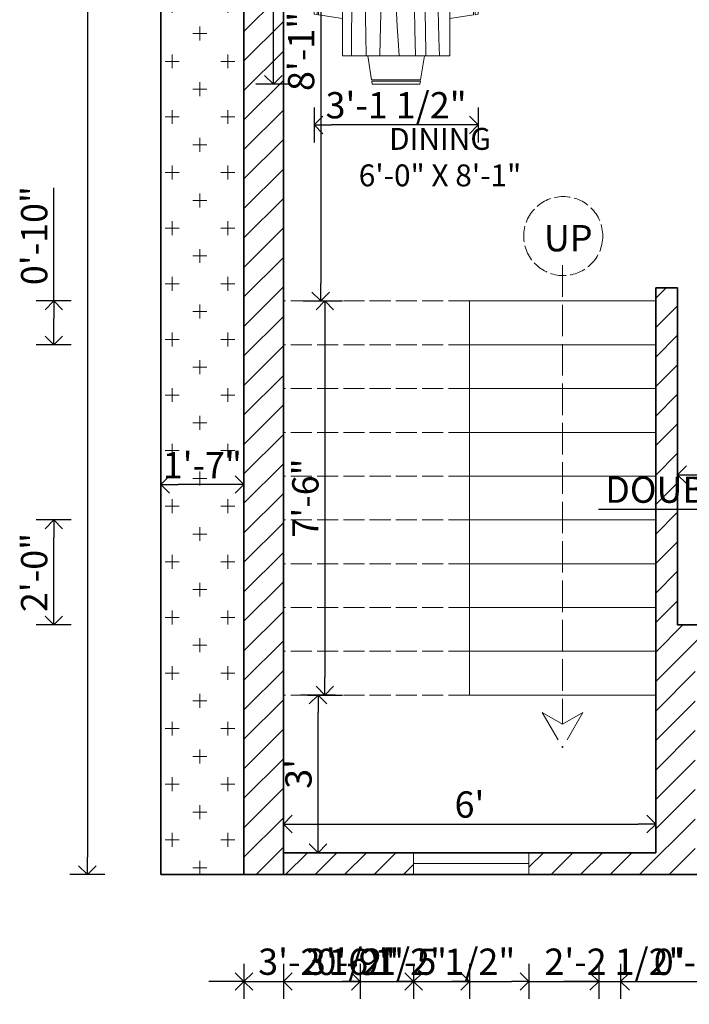
# Model space of a CAD drawing. Units: inches. Extents: x 686 to 1065, y 83 to 664.
# Tile 1 of 5: x 691 to 844, y 83 to 308. Entities that reach past the tile are written whole.
import ezdxf

# ---------------------------------------------------------------- set-up
doc = ezdxf.new("R2010")
doc.units = ezdxf.units.IN
doc.linetypes.add('ACAD_ISO02W100', pattern=[15, 12, -3])
for name, color, linetype, lineweight in [('A-ANNO-DIMS', 2, 'Continuous', 18), ('A-ANNO-SYMB', 253, 'ACAD_ISO02W100', 18), ('A-ANNO-TEXT', 7, 'Continuous', 20), ('A-AREA-IDEN', 7, 'Continuous', 20), ('A-FLOR-STRS', 7, 'Continuous', 20), ('A-FLOR-STRS-OVHD', 253, 'ACAD_ISO02W100', 18), ('A-FURN', 8, 'Continuous', 18), ('A-GLAZ', 172, 'Continuous', 18), ('A-WALL', 7, 'Continuous', 35), ('A-WALL-PATT', 253, 'Continuous', 13), ('C-PROP', 7, 'Continuous', 35), ('L-SITE-PATT', 94, 'Continuous', 13)]:
    doc.layers.add(name, color=color, linetype=linetype, lineweight=lineweight)
doc.styles.get("Standard").update_dxf_attribs({"font": 'arial.ttf'})
doc.dimstyles.new('ISO-25', dxfattribs={"dimtxt": 6, "dimasz": 4, "dimexe": 4, "dimexo": 4, "dimtad": 1, "dimdec": 1, "dimlunit": 3, "dimtxsty": 'Standard', "dimblk": 'OPEN90', "dimcen": 2.5, "dimadec": 0, "dimazin": 0, "dimtfac": 1, "dimtdec": 1, "dimtmove": 0, "dimatfit": 3, "dimfxl": 4, "dimfxlon": 1, "dimarcsym": 0})

# ---------------------------------------------------------------- blocks, each defined once
blk = doc.blocks.new('_Open90')
at = {"color": 0, "linetype": 'ByBlock', "lineweight": -2}
for p, q in [((0, 0), (-1, 0)), ((-0.5, 0.5), (0, 0)), ((0, 0), (-0.5, -0.5))]:
    blk.add_line(p, q, dxfattribs=at)
blk = doc.blocks.new('*D12')
at = {"layer": 'A-ANNO-DIMS', "color": 0, "lineweight": -2, "transparency": 16777216}
for p, q in [((723.37, 201.81), (723.37, 205.81)), ((742.37, 201.81), (742.37, 205.81)), ((738.37, 201.81), (727.37, 201.81))]:
    blk.add_line(p, q, dxfattribs=at)
at = {"layer": 'Defpoints', "color": 0, "transparency": 16777216}
for p in [(723.37, 201.81), (723.37, 201.25), (742.37, 201.25)]:
    blk.add_point(p, dxfattribs=at)
at = {"layer": 'A-ANNO-DIMS', "color": 0, "lineweight": -2, "transparency": 16777216, "xscale": 4, "yscale": 4, "zscale": 4, "rotation": 180}
blk.add_blockref('_Open90', (723.37, 201.81), dxfattribs=at)
at = {"layer": 'A-ANNO-DIMS', "color": 0, "lineweight": -2, "transparency": 16777216, "xscale": 4, "yscale": 4, "zscale": 4}
blk.add_blockref('_Open90', (742.37, 201.81), dxfattribs=at)
at = {"layer": 'A-ANNO-DIMS', "color": 0, "transparency": 16777216, "insert": (732.87, 205.45), "char_height": 6, "attachment_point": 5}
blk.add_mtext('1\'-7"', dxfattribs=at)
blk = doc.blocks.new('*D13')
at = {"layer": 'A-ANNO-DIMS', "color": 0, "lineweight": -2, "transparency": 16777216}
for p, q in [((755.89, 357.73), (763.89, 357.73)), ((759.89, 353.73), (759.89, 247.73)), ((755.89, 243.73), (763.89, 243.73))]:
    blk.add_line(p, q, dxfattribs=at)
at = {"layer": 'Defpoints', "color": 0, "transparency": 16777216}
for p in [(751.37, 357.73), (751.37, 243.73), (759.89, 243.73)]:
    blk.add_point(p, dxfattribs=at)
at = {"layer": 'A-ANNO-DIMS', "color": 0, "lineweight": -2, "transparency": 16777216, "xscale": 4, "yscale": 4, "zscale": 4}
for p, rotation in [((759.89, 357.73), 90), ((759.89, 243.73), 270)]:
    blk.add_blockref('_Open90', p, dxfattribs=dict(at, rotation=rotation))
at = {"layer": 'A-ANNO-DIMS', "color": 0, "transparency": 16777216, "insert": (756.2, 300.73), "char_height": 6, "attachment_point": 5, "rotation": 90}
blk.add_mtext('8\'-1"', dxfattribs=at)
blk = doc.blocks.new('*D14')
at = {"layer": 'A-ANNO-DIMS', "color": 0, "lineweight": -2, "transparency": 16777216}
for p, q in [((763.29, 153.73), (755.29, 153.73)), ((759.29, 121.73), (759.29, 149.73)), ((763.29, 117.73), (755.29, 117.73))]:
    blk.add_line(p, q, dxfattribs=at)
at = {"layer": 'Defpoints', "color": 0, "transparency": 16777216}
for p in [(759.29, 153.73), (836.37, 153.73), (836.37, 117.73)]:
    blk.add_point(p, dxfattribs=at)
at = {"layer": 'A-ANNO-DIMS', "color": 0, "lineweight": -2, "transparency": 16777216, "xscale": 4, "yscale": 4, "zscale": 4}
for p, rotation in [((759.29, 153.73), 90), ((759.29, 117.73), 270)]:
    blk.add_blockref('_Open90', p, dxfattribs=dict(at, rotation=rotation))
at = {"layer": 'A-ANNO-DIMS', "color": 0, "transparency": 16777216, "insert": (755.6, 135.73), "char_height": 6, "attachment_point": 5, "rotation": 90}
blk.add_mtext("3'", dxfattribs=at)
blk = doc.blocks.new('*D15')
at = {"layer": 'A-ANNO-DIMS', "color": 0, "lineweight": -2, "transparency": 16777216}
for p, q in [((751.37, 121.73), (751.37, 128.26)), ((836.37, 121.73), (836.37, 128.26)), ((755.37, 124.26), (832.37, 124.26))]:
    blk.add_line(p, q, dxfattribs=at)
at = {"layer": 'Defpoints', "color": 0, "transparency": 16777216}
for p in [(836.37, 124.26), (751.37, 117.73), (836.37, 117.73)]:
    blk.add_point(p, dxfattribs=at)
at = {"layer": 'A-ANNO-DIMS', "color": 0, "lineweight": -2, "transparency": 16777216, "xscale": 4, "yscale": 4, "zscale": 4, "rotation": 180}
blk.add_blockref('_Open90', (751.37, 124.26), dxfattribs=at)
at = {"layer": 'A-ANNO-DIMS', "color": 0, "lineweight": -2, "transparency": 16777216, "xscale": 4, "yscale": 4, "zscale": 4}
blk.add_blockref('_Open90', (836.37, 124.26), dxfattribs=at)
at = {"layer": 'A-ANNO-DIMS', "color": 0, "transparency": 16777216, "insert": (793.87, 127.95), "char_height": 6, "attachment_point": 5}
blk.add_mtext("6'", dxfattribs=at)
blk = doc.blocks.new('*D16')
at = {"layer": 'A-ANNO-DIMS', "color": 0, "lineweight": -2, "transparency": 16777216}
for p, q in [((756.85, 243.73), (764.85, 243.73)), ((760.85, 239.73), (760.85, 157.73)), ((756.85, 153.73), (764.85, 153.73))]:
    blk.add_line(p, q, dxfattribs=at)
at = {"layer": 'Defpoints', "color": 0, "transparency": 16777216}
for p in [(751.37, 243.73), (751.37, 153.73), (760.85, 153.73)]:
    blk.add_point(p, dxfattribs=at)
at = {"layer": 'A-ANNO-DIMS', "color": 0, "lineweight": -2, "transparency": 16777216, "xscale": 4, "yscale": 4, "zscale": 4}
for p, rotation in [((760.85, 243.73), 90), ((760.85, 153.73), 270)]:
    blk.add_blockref('_Open90', p, dxfattribs=dict(at, rotation=rotation))
at = {"layer": 'A-ANNO-DIMS', "color": 0, "transparency": 16777216, "insert": (757.17, 198.73), "char_height": 6, "attachment_point": 5, "rotation": 90}
blk.add_mtext('7\'-6"', dxfattribs=at)
blk = doc.blocks.new('Dining Set - 36 x 72 in.')
for p, q in [((-22, 27.5), (-22.1562, 26.50042)), ((-5.8416, 26.5), (-22.1534, 26.5)), ((-22, 27.5), (-6, 27.5)), ((-5.8437, 26.49966), (-6, 27.5)), ((6, 27.5), (5.8438, 26.50042)), ((22.1584, 26.5), (5.8466, 26.5)), ((6, 27.5), (22, 27.5)), ((22.1563, 26.49966), (22, 27.5)), ((-22.2343, 26.00059), (-23.4847, 17.99762)), ((-22.2304, 26), (-5.7608, 26)), ((-4.5152, 17.99762), (-5.7655, 25.99926)), ((5.7657, 26.00059), (4.5153, 17.99762)), ((5.7696, 26), (22.2392, 26)), ((23.4848, 17.99762), (22.2345, 25.99926)), ((36, 18), (-36, 18)), ((-36, 18), (-36, -18)), ((36, -18), (36, 18)), ((-45.5, 8), (-44.5004, 8.15617)), ((-45.5, 8), (-45.5, -8)), ((-44.5, -8.15843), (-44.5, 8.15338)), ((-44.0006, 8.23428), (-35.9976, 9.48474)), ((-44, 8.23041), (-44, -8.23915)), ((44.0006, 8.23428), (35.9976, 9.48474)), ((44, 8.23041), (44, -8.23915)), ((44.5, -8.15843), (44.5, 8.15338)), ((45.5, 8), (44.5005, 8.15617)), ((45.5, 8), (45.5, -8)), ((-44.4997, -8.15631), (-45.5, -8)), ((-35.9976, -9.48476), (-43.9993, -8.2345)), ((35.9976, -9.48476), (43.9993, -8.2345)), ((44.4997, -8.15631), (45.5, -8)), ((-36, -18), (36, -18)), ((-22.2343, -26.0006), (-23.4847, -17.99762)), ((-4.5152, -17.99762), (-5.7655, -25.99928)), ((5.7657, -26.0006), (4.5153, -17.99762)), ((23.4848, -17.99762), (22.2345, -25.99928)), ((-22.2304, -26), (-5.7608, -26)), ((5.7696, -26), (22.2392, -26)), ((-22, -27.5), (-22.1562, -26.50044)), ((-5.8416, -26.5), (-22.1534, -26.5)), ((-22, -27.5), (-6, -27.5)), ((-5.8437, -26.49967), (-6, -27.5)), ((6, -27.5), (5.8438, -26.50044)), ((22.1584, -26.5), (5.8466, -26.5)), ((6, -27.5), (22, -27.5)), ((22.1563, -26.49967), (22, -27.5))]:
    blk.add_line(p, q)
for points in [[(-36, 15), (-31.1772, 14.97754), (-26.8079, 14.91406), (-22.8538, 14.81543), (-19.276, 14.6875), (-16.0362, 14.53613), (-13.0957, 14.36718), (-10.4159, 14.18652), (-7.9583, 14), (-5.6904, 13.81315), (-3.6035, 13.63021), (-1.6954, 13.45508), (0.0365, 13.29166), (1.5945, 13.14388), (2.9811, 13.01562), (4.1988, 12.9108), (5.25, 12.83333), (6.1393, 12.78613), (6.8802, 12.76823), (7.4883, 12.77767), (7.9792, 12.8125), (8.3685, 12.87077), (8.6719, 12.95052), (8.9049, 13.0498), (9.0833, 13.16666), (9.2205, 13.29899), (9.3216, 13.44401), (9.3895, 13.59879), (9.4271, 13.76041), (9.4373, 13.92594), (9.4232, 14.09245), (9.3875, 14.257), (9.3333, 14.41666), (9.2638, 14.56917), (9.1836, 14.71484), (9.0975, 14.85465), (9.0104, 14.98958), (8.9272, 15.1206), (8.8529, 15.2487), (8.7922, 15.37483), (8.75, 15.5), (8.7305, 15.62467), (8.7344, 15.74739), (8.7617, 15.86621), (8.8125, 15.97916), (8.8867, 16.08431), (8.9844, 16.17968), (9.1055, 16.26334), (9.25, 16.33333), (9.4189, 16.38802), (9.6172, 16.42708), (9.8506, 16.45052), (10.125, 16.45833), (10.4463, 16.45052), (10.8203, 16.42708), (11.2529, 16.38802), (11.75, 16.33333), (12.3184, 16.26318), (12.9694, 16.17838), (13.7151, 16.07991), (14.5677, 15.96875), (15.5395, 15.84586), (16.6426, 15.71224), (17.8893, 15.56884), (19.2917, 15.41666), (20.859, 15.25667), (22.5879, 15.08984), (24.4721, 14.91715), (26.5052, 14.73958), (28.6809, 14.5581), (30.9929, 14.3737), (33.4347, 14.18733), (36, 14)], [(-36, 10), (-28.9766, 10.14274), (-23.1725, 10.20442), (-18.4241, 10.19775), (-14.5677, 10.13541), (-11.4399, 10.03011), (-8.877, 9.89453), (-6.7154, 9.74137), (-4.7917, 9.58333), (-2.9698, 9.43082), (-1.2246, 9.28515), (0.4415, 9.14534), (2.026, 9.01041), (3.5266, 8.87939), (4.9408, 8.7513), (6.266, 8.62516), (7.5, 8.5), (8.6411, 8.37549), (9.6914, 8.2539), (10.6538, 8.13818), (11.5312, 8.03125), (12.3267, 7.93603), (13.043, 7.85547), (13.6831, 7.79248), (14.25, 7.75), (14.7471, 7.7303), (15.1797, 7.73307), (15.5537, 7.75732), (15.875, 7.80208), (16.1494, 7.86637), (16.3828, 7.94922), (16.5811, 8.04964), (16.75, 8.16666), (16.8944, 8.29915), (17.0143, 8.44531), (17.1089, 8.60319), (17.1771, 8.77083), (17.218, 8.94629), (17.2305, 9.1276), (17.2137, 9.31282), (17.1667, 9.5), (17.0895, 9.6875), (16.987, 9.875), (16.8649, 10.0625), (16.7292, 10.25), (16.5856, 10.4375), (16.4401, 10.625), (16.2985, 10.8125), (16.1667, 11), (16.05, 11.18733), (15.9518, 11.3737), (15.8752, 11.5581), (15.8229, 11.73958), (15.798, 11.91715), (15.8034, 12.08984), (15.842, 12.25667), (15.9167, 12.41666), (16.0295, 12.56836), (16.1784, 12.70833), (16.3605, 12.83268), (16.5729, 12.9375), (16.8127, 13.01888), (17.0768, 13.07291), (17.3625, 13.0957), (17.6667, 13.08333), (17.9894, 13.03312), (18.3418, 12.94726), (18.7382, 12.82918), (19.1927, 12.68229), (19.7195, 12.51001), (20.3327, 12.31575), (21.0465, 12.10294), (21.875, 11.875), (22.8357, 11.63354), (23.959, 11.37304), (25.2786, 11.08618), (26.8282, 10.76562), (28.6414, 10.40405), (30.752, 9.99414), (33.1936, 9.52856), (36, 9)], [(-36, 5.5), (-30.7157, 5.3348), (-26.069, 5.20963), (-21.9946, 5.11767), (-18.4271, 5.05208), (-15.3009, 5.00602), (-12.5508, 4.97265), (-10.1112, 4.94515), (-7.9167, 4.91666), (-5.909, 4.88167), (-4.0586, 4.83984), (-2.3429, 4.79215), (-0.7396, 4.73958), (0.7739, 4.6831), (2.22, 4.6237), (3.6213, 4.56233), (5, 4.5), (6.373, 4.43782), (7.7344, 4.3776), (9.0723, 4.32129), (10.375, 4.27083), (11.6309, 4.22819), (12.8281, 4.19531), (13.9551, 4.17415), (15, 4.16666), (15.954, 4.17448), (16.819, 4.19791), (17.6001, 4.23698), (18.3021, 4.29166), (18.9299, 4.36198), (19.4883, 4.44791), (19.9823, 4.54948), (20.4167, 4.66666), (20.7969, 4.79899), (21.1302, 4.94401), (21.4245, 5.09879), (21.6875, 5.26041), (21.9271, 5.42594), (22.1511, 5.59245), (22.3672, 5.757), (22.5834, 5.91666), (22.8065, 6.06868), (23.0404, 6.21093), (23.2879, 6.34147), (23.5521, 6.45833), (23.8358, 6.55957), (24.142, 6.64323), (24.4735, 6.70735), (24.8334, 6.75), (25.2235, 6.76969), (25.642, 6.76692), (26.0858, 6.74267), (26.5521, 6.69791), (27.0379, 6.63362), (27.5404, 6.55078), (28.0565, 6.45036), (28.5834, 6.33333), (29.1242, 6.19987), (29.7071, 6.04687), (30.3661, 5.87044), (31.1354, 5.66666), (32.0493, 5.43164), (33.142, 5.16146), (34.4475, 4.85221), (36, 4.5)], [(-36, -1), (-30.7915, -0.6591), (-26.0195, -0.38216), (-21.6519, -0.16284), (-17.6563, 0.00521), (-14.0005, 0.12833), (-10.6523, 0.21289), (-7.5796, 0.26522), (-4.75, 0.29166), (-2.134, 0.29793), (0.2878, 0.28711), (2.5317, 0.26163), (4.6146, 0.22396), (6.5529, 0.17651), (8.3633, 0.12174), (10.0623, 0.06209), (11.6667, 0), (13.1899, -0.06201), (14.6341, -0.1211), (15.9982, -0.17432), (17.2813, -0.21875), (18.4823, -0.25147), (19.6003, -0.26953), (20.6343, -0.27002), (21.5834, -0.25), (22.4481, -0.20768), (23.2357, -0.14584), (23.9549, -0.06836), (24.6146, 0.02083), (25.2235, 0.11784), (25.7904, 0.21875), (26.3241, 0.31966), (26.8334, 0.41666), (27.3265, 0.50618), (27.8099, 0.58593), (28.2894, 0.65397), (28.7709, 0.70833), (29.2601, 0.74707), (29.763, 0.76823), (30.2855, 0.76985), (30.8334, 0.75), (31.4088, 0.70784), (31.9994, 0.64713), (32.589, 0.57275), (33.1615, 0.48958), (33.7008, 0.4025), (34.1908, 0.3164), (34.6153, 0.23616), (34.9584, 0.16666), (35.2099, 0.11165), (35.3848, 0.07031), (35.504, 0.04069), (35.5886, 0.02083), (35.6594, 0.00879), (35.7377, 0.0026), (35.8442, 0.00032), (36, 0)], [(-36, -6.5), (-27.1843, -6.31267), (-20.084, -6.1263), (-14.469, -5.9419), (-10.1094, -5.76042), (-6.7752, -5.58285), (-4.2363, -5.41016), (-2.2629, -5.24333), (-0.625, -5.08334), (0.8708, -4.93099), (2.2715, -4.78646), (3.5872, -4.64974), (4.8281, -4.52084), (6.0046, -4.39974), (7.127, -4.28646), (8.2053, -4.18099), (9.25, -4.08334), (10.2705, -3.99382), (11.2734, -3.91407), (12.2647, -3.84603), (13.25, -3.79167), (14.2354, -3.75293), (15.2266, -3.73177), (16.2295, -3.73015), (17.25, -3.75), (18.2912, -3.79248), (19.3451, -3.85547), (20.4009, -3.93604), (21.4479, -4.03125), (22.4754, -4.13819), (23.4727, -4.25391), (24.4289, -4.37549), (25.3334, -4.5), (26.1785, -4.62492), (26.9694, -4.74935), (27.7145, -4.87281), (28.4219, -4.99479), (29.1, -5.11483), (29.7572, -5.23242), (30.4016, -5.34709), (31.0417, -5.45834), (31.6837, -5.56437), (32.3262, -5.65821), (32.9658, -5.73153), (33.599, -5.77604), (34.2224, -5.78345), (34.8327, -5.74545), (35.4264, -5.65373), (36, -5.5)], [(-36, -10), (-26.4022, -9.81299), (-18.4675, -9.62891), (-11.9839, -9.45069), (-6.7396, -9.28125), (-2.5226, -9.12354), (0.8789, -8.98047), (3.6769, -8.85498), (6.0833, -8.75), (8.2767, -8.66765), (10.3021, -8.60677), (12.1712, -8.56543), (13.8958, -8.54167), (15.4876, -8.53353), (16.9583, -8.53907), (18.3197, -8.55632), (19.5834, -8.58334), (20.7616, -8.61841), (21.8685, -8.66081), (22.9188, -8.71004), (23.9271, -8.76563), (24.9081, -8.82707), (25.8763, -8.89388), (26.8465, -8.96558), (27.8334, -9.04167), (28.8474, -9.12118), (29.8828, -9.20117), (30.93, -9.27824), (31.9792, -9.34896), (33.0205, -9.40991), (34.0443, -9.45768), (35.0407, -9.48885), (36, -9.5)], [(-36, -14.5), (-30.0881, -14.33513), (-25.0332, -14.21224), (-20.7312, -14.12647), (-17.0781, -14.07292), (-13.97, -14.04671), (-11.3027, -14.04297), (-8.9724, -14.05681), (-6.875, -14.08334), (-4.9224, -14.11833), (-3.0905, -14.16016), (-1.3709, -14.20785), (0.2448, -14.26042), (1.7647, -14.3169), (3.1973, -14.3763), (4.5507, -14.43767), (5.8333, -14.5), (7.0554, -14.5621), (8.235, -14.62175), (9.3922, -14.67652), (10.5469, -14.72396), (11.7192, -14.76164), (12.929, -14.78711), (14.1965, -14.79794), (15.5417, -14.79167), (16.9933, -14.76424), (18.6152, -14.70508), (20.4804, -14.60197), (22.6615, -14.44271), (25.2312, -14.21509), (28.2624, -13.9069), (31.8277, -13.50594), (36, -13)]]:
    blk.add_lwpolyline(points)
blk = doc.blocks.new('*D19')
at = {"layer": 'A-ANNO-DIMS', "color": 0, "lineweight": -2, "transparency": 16777216}
for p, q in [((841.37, 203.96), (841.37, 208.06)), ((889.37, 203.96), (889.37, 208.06)), ((845.37, 204.06), (885.37, 204.06))]:
    blk.add_line(p, q, dxfattribs=at)
at = {"layer": 'Defpoints', "color": 0, "transparency": 16777216}
for p in [(889.37, 204.06), (841.37, 199.96), (889.37, 199.96)]:
    blk.add_point(p, dxfattribs=at)
at = {"layer": 'A-ANNO-DIMS', "color": 0, "lineweight": -2, "transparency": 16777216, "xscale": 4, "yscale": 4, "zscale": 4, "rotation": 180}
blk.add_blockref('_Open90', (841.37, 204.06), dxfattribs=at)
at = {"layer": 'A-ANNO-DIMS', "color": 0, "lineweight": -2, "transparency": 16777216, "xscale": 4, "yscale": 4, "zscale": 4}
blk.add_blockref('_Open90', (889.37, 204.06), dxfattribs=at)
at = {"layer": 'A-ANNO-DIMS', "color": 0, "transparency": 16777216, "insert": (865.37, 207.68), "char_height": 6, "attachment_point": 5}
blk.add_mtext("4'", dxfattribs=at)
blk = doc.blocks.new('*D18')
at = {"layer": 'A-ANNO-DIMS', "color": 0, "lineweight": -2, "transparency": 16777216}
for p, q in [((710.63, 592.73), (702.63, 592.73)), ((706.63, 588.73), (706.63, 116.73)), ((710.63, 112.73), (702.63, 112.73))]:
    blk.add_line(p, q, dxfattribs=at)
at = {"layer": 'Defpoints', "color": 0, "transparency": 16777216}
for p in [(723.37, 592.73), (706.63, 112.73), (723.37, 112.73)]:
    blk.add_point(p, dxfattribs=at)
at = {"layer": 'A-ANNO-DIMS', "color": 0, "lineweight": -2, "transparency": 16777216, "xscale": 4, "yscale": 4, "zscale": 4}
for p, rotation in [((706.63, 592.73), 90), ((706.63, 112.73), 270)]:
    blk.add_blockref('_Open90', p, dxfattribs=dict(at, rotation=rotation))
at = {"layer": 'A-ANNO-DIMS', "color": 0, "transparency": 16777216, "insert": (702.94, 352.73), "char_height": 6, "attachment_point": 5, "rotation": 90}
blk.add_mtext("40'", dxfattribs=at)
blk = doc.blocks.new('*D34')
at = {"layer": 'A-ANNO-DIMS', "color": 0, "lineweight": -2, "transparency": 16777216}
for p, q in [((749.09, 355.19), (749.09, 426.38)), ((753.09, 355.19), (745.09, 355.19)), ((749.09, 297.22), (749.09, 351.19)), ((753.09, 293.22), (745.09, 293.22))]:
    blk.add_line(p, q, dxfattribs=at)
at = {"layer": 'Defpoints', "color": 0, "transparency": 16777216}
for p in [(749.09, 355.19), (758.38, 355.19), (758.38, 293.22)]:
    blk.add_point(p, dxfattribs=at)
at = {"layer": 'A-ANNO-DIMS', "color": 0, "lineweight": -2, "transparency": 16777216, "xscale": 4, "yscale": 4, "zscale": 4}
for p, rotation in [((749.09, 355.19), 90), ((749.09, 293.22), 270)]:
    blk.add_blockref('_Open90', p, dxfattribs=dict(at, rotation=rotation))
at = {"layer": 'A-ANNO-DIMS', "color": 0, "transparency": 16777216, "insert": (745.36, 392.78), "char_height": 6, "attachment_point": 5, "rotation": 90}
blk.add_mtext('DINING SET 5\'-2"', dxfattribs=at)
blk = doc.blocks.new('*D35')
at = {"layer": 'A-ANNO-DIMS', "color": 0, "lineweight": -2, "transparency": 16777216}
for p, q in [((758.38, 287.93), (758.38, 279.93)), ((795.83, 287.93), (795.83, 279.93)), ((791.83, 283.93), (762.38, 283.93))]:
    blk.add_line(p, q, dxfattribs=at)
at = {"layer": 'Defpoints', "color": 0, "transparency": 16777216}
for p in [(758.38, 293.22), (795.83, 293.22), (758.38, 283.93)]:
    blk.add_point(p, dxfattribs=at)
at = {"layer": 'A-ANNO-DIMS', "color": 0, "lineweight": -2, "transparency": 16777216, "xscale": 4, "yscale": 4, "zscale": 4, "rotation": 180}
blk.add_blockref('_Open90', (758.38, 283.93), dxfattribs=at)
at = {"layer": 'A-ANNO-DIMS', "color": 0, "lineweight": -2, "transparency": 16777216, "xscale": 4, "yscale": 4, "zscale": 4}
blk.add_blockref('_Open90', (795.83, 283.93), dxfattribs=at)
at = {"layer": 'A-ANNO-DIMS', "color": 0, "transparency": 16777216, "insert": (777.11, 287.66), "char_height": 6, "attachment_point": 5}
blk.add_mtext('3\'-1 1/2"', dxfattribs=at)
blk = doc.blocks.new('*D40')
at = {"layer": 'A-ANNO-DIMS', "color": 0, "lineweight": -2, "transparency": 16777216}
for p, q in [((902.89, 194.73), (902.89, 200.13)), ((938.89, 194.73), (938.89, 200.13)), ((902.89, 196.13), (823.3, 196.13)), ((934.89, 196.13), (906.89, 196.13))]:
    blk.add_line(p, q, dxfattribs=at)
at = {"layer": 'Defpoints', "color": 0, "transparency": 16777216}
for p in [(902.89, 196.13), (902.89, 190.73), (938.89, 190.73)]:
    blk.add_point(p, dxfattribs=at)
at = {"layer": 'A-ANNO-DIMS', "color": 0, "lineweight": -2, "transparency": 16777216, "xscale": 4, "yscale": 4, "zscale": 4, "rotation": 180}
blk.add_blockref('_Open90', (902.89, 196.13), dxfattribs=at)
at = {"layer": 'A-ANNO-DIMS', "color": 0, "lineweight": -2, "transparency": 16777216, "xscale": 4, "yscale": 4, "zscale": 4}
blk.add_blockref('_Open90', (938.89, 196.13), dxfattribs=at)
at = {"layer": 'A-ANNO-DIMS', "color": 0, "transparency": 16777216, "insert": (861.09, 199.86), "char_height": 6, "attachment_point": 5}
blk.add_mtext('DOUBLE SINK 3\'-0"', dxfattribs=at)
blk = doc.blocks.new('*D59')
at = {"layer": 'A-ANNO-DIMS', "color": 0, "lineweight": -2, "transparency": 16777216}
for p, q in [((742.37, 92.32), (742.37, 84.32)), ((781.1, 92.32), (781.1, 84.32)), ((746.37, 88.32), (777.1, 88.32))]:
    blk.add_line(p, q, dxfattribs=at)
at = {"layer": 'Defpoints', "color": 0, "transparency": 16777216}
for p in [(742.37, 112.73), (781.1, 112.73), (781.1, 88.32)]:
    blk.add_point(p, dxfattribs=at)
at = {"layer": 'A-ANNO-DIMS', "color": 0, "lineweight": -2, "transparency": 16777216, "xscale": 4, "yscale": 4, "zscale": 4, "rotation": 180}
blk.add_blockref('_Open90', (742.37, 88.32), dxfattribs=at)
at = {"layer": 'A-ANNO-DIMS', "color": 0, "lineweight": -2, "transparency": 16777216, "xscale": 4, "yscale": 4, "zscale": 4}
blk.add_blockref('_Open90', (781.1, 88.32), dxfattribs=at)
at = {"layer": 'A-ANNO-DIMS', "color": 0, "transparency": 16777216, "insert": (761.73, 92.05), "char_height": 6, "attachment_point": 5}
blk.add_mtext('3\'-2 1/2"', dxfattribs=at)
blk = doc.blocks.new('*D60')
at = {"layer": 'A-ANNO-DIMS', "color": 0, "lineweight": -2, "transparency": 16777216}
for p, q in [((781.1, 92.32), (781.1, 84.32)), ((807.43, 92.32), (807.43, 84.32)), ((785.1, 88.32), (803.43, 88.32)), ((807.43, 88.32), (842.71, 88.32))]:
    blk.add_line(p, q, dxfattribs=at)
at = {"layer": 'Defpoints', "color": 0, "transparency": 16777216}
for p in [(781.1, 112.73), (807.43, 112.73), (807.43, 88.32)]:
    blk.add_point(p, dxfattribs=at)
at = {"layer": 'A-ANNO-DIMS', "color": 0, "lineweight": -2, "transparency": 16777216, "xscale": 4, "yscale": 4, "zscale": 4, "rotation": 180}
blk.add_blockref('_Open90', (781.1, 88.32), dxfattribs=at)
at = {"layer": 'A-ANNO-DIMS', "color": 0, "lineweight": -2, "transparency": 16777216, "xscale": 4, "yscale": 4, "zscale": 4}
blk.add_blockref('_Open90', (807.43, 88.32), dxfattribs=at)
at = {"layer": 'A-ANNO-DIMS', "color": 0, "transparency": 16777216, "insert": (827.07, 92.05), "char_height": 6, "attachment_point": 5}
blk.add_mtext('2\'-2 1/2"', dxfattribs=at)
blk = doc.blocks.new('*D62')
at = {"layer": 'A-ANNO-DIMS', "color": 0, "lineweight": -2, "transparency": 16777216}
for p, q in [((742.37, 92.32), (742.37, 84.32)), ((751.37, 92.32), (751.37, 84.32)), ((738.37, 88.32), (734.37, 88.32)), ((742.37, 88.32), (751.37, 88.32)), ((755.37, 88.32), (776.57, 88.32))]:
    blk.add_line(p, q, dxfattribs=at)
at = {"layer": 'Defpoints', "color": 0, "transparency": 16777216}
for p in [(742.37, 376.23), (751.37, 376.23), (751.37, 88.32)]:
    blk.add_point(p, dxfattribs=at)
at = {"layer": 'A-ANNO-DIMS', "color": 0, "lineweight": -2, "transparency": 16777216, "xscale": 4, "yscale": 4, "zscale": 4}
blk.add_blockref('_Open90', (742.37, 88.32), dxfattribs=at)
at = {"layer": 'A-ANNO-DIMS', "color": 0, "lineweight": -2, "transparency": 16777216, "xscale": 4, "yscale": 4, "zscale": 4, "rotation": 180}
blk.add_blockref('_Open90', (751.37, 88.32), dxfattribs=at)
at = {"layer": 'A-ANNO-DIMS', "color": 0, "transparency": 16777216, "insert": (767.97, 92.01), "char_height": 6, "attachment_point": 5}
blk.add_mtext('0\'-9"', dxfattribs=at)
blk = doc.blocks.new('*D63')
at = {"layer": 'A-ANNO-DIMS', "color": 0, "lineweight": -2, "transparency": 16777216}
for p, q in [((823.37, 92.32), (823.37, 84.32)), ((828.37, 92.32), (828.37, 84.32)), ((819.37, 88.32), (815.37, 88.32)), ((823.37, 88.32), (828.37, 88.32)), ((832.37, 88.32), (853.57, 88.32))]:
    blk.add_line(p, q, dxfattribs=at)
at = {"layer": 'Defpoints', "color": 0, "transparency": 16777216}
for p in [(823.37, 362.73), (828.37, 357.73), (828.37, 88.32)]:
    blk.add_point(p, dxfattribs=at)
at = {"layer": 'A-ANNO-DIMS', "color": 0, "lineweight": -2, "transparency": 16777216, "xscale": 4, "yscale": 4, "zscale": 4}
blk.add_blockref('_Open90', (823.37, 88.32), dxfattribs=at)
at = {"layer": 'A-ANNO-DIMS', "color": 0, "lineweight": -2, "transparency": 16777216, "xscale": 4, "yscale": 4, "zscale": 4, "rotation": 180}
blk.add_blockref('_Open90', (828.37, 88.32), dxfattribs=at)
at = {"layer": 'A-ANNO-DIMS', "color": 0, "transparency": 16777216, "insert": (844.97, 92.01), "char_height": 6, "attachment_point": 5}
blk.add_mtext('0\'-5"', dxfattribs=at)
blk = doc.blocks.new('*D67')
at = {"layer": 'A-ANNO-DIMS', "color": 0, "lineweight": -2, "transparency": 16777216}
for p, q in [((698.96, 243.73), (698.96, 269.59)), ((702.96, 243.73), (694.96, 243.73)), ((698.96, 237.73), (698.96, 239.73)), ((702.96, 233.73), (694.96, 233.73))]:
    blk.add_line(p, q, dxfattribs=at)
at = {"layer": 'Defpoints', "color": 0, "transparency": 16777216}
for p in [(698.96, 243.73), (751.37, 243.73), (751.37, 233.73)]:
    blk.add_point(p, dxfattribs=at)
at = {"layer": 'A-ANNO-DIMS', "color": 0, "lineweight": -2, "transparency": 16777216, "xscale": 4, "yscale": 4, "zscale": 4}
for p, rotation in [((698.96, 243.73), 90), ((698.96, 233.73), 270)]:
    blk.add_blockref('_Open90', p, dxfattribs=dict(at, rotation=rotation))
at = {"layer": 'A-ANNO-DIMS', "color": 0, "transparency": 16777216, "insert": (695.27, 258.66), "char_height": 6, "attachment_point": 5, "rotation": 90}
blk.add_mtext('0\'-10"', dxfattribs=at)
blk = doc.blocks.new('*D68')
at = {"layer": 'A-ANNO-DIMS', "color": 0, "lineweight": -2, "transparency": 16777216}
for p, q in [((751.37, 92.32), (751.37, 84.32)), ((793.87, 92.32), (793.87, 84.32)), ((755.37, 88.32), (789.87, 88.32))]:
    blk.add_line(p, q, dxfattribs=at)
at = {"layer": 'Defpoints', "color": 0, "transparency": 16777216}
for p in [(751.37, 153.73), (793.87, 153.73), (793.87, 88.32)]:
    blk.add_point(p, dxfattribs=at)
at = {"layer": 'A-ANNO-DIMS', "color": 0, "lineweight": -2, "transparency": 16777216, "xscale": 4, "yscale": 4, "zscale": 4, "rotation": 180}
blk.add_blockref('_Open90', (751.37, 88.32), dxfattribs=at)
at = {"layer": 'A-ANNO-DIMS', "color": 0, "lineweight": -2, "transparency": 16777216, "xscale": 4, "yscale": 4, "zscale": 4}
blk.add_blockref('_Open90', (793.87, 88.32), dxfattribs=at)
at = {"layer": 'A-ANNO-DIMS', "color": 0, "transparency": 16777216, "insert": (772.62, 92.05), "char_height": 6, "attachment_point": 5}
blk.add_mtext('3\'-6 1/2"', dxfattribs=at)
blk = doc.blocks.new('*D70')
at = {"layer": 'A-ANNO-DIMS', "color": 0, "lineweight": -2, "transparency": 16777216}
for p, q in [((702.96, 193.73), (694.96, 193.73)), ((698.96, 173.73), (698.96, 189.73)), ((702.96, 169.73), (694.96, 169.73))]:
    blk.add_line(p, q, dxfattribs=at)
at = {"layer": 'Defpoints', "color": 0, "transparency": 16777216}
for p in [(698.96, 193.73), (894.37, 193.73), (894.37, 169.73)]:
    blk.add_point(p, dxfattribs=at)
at = {"layer": 'A-ANNO-DIMS', "color": 0, "lineweight": -2, "transparency": 16777216, "xscale": 4, "yscale": 4, "zscale": 4}
for p, rotation in [((698.96, 193.73), 90), ((698.96, 169.73), 270)]:
    blk.add_blockref('_Open90', p, dxfattribs=dict(at, rotation=rotation))
at = {"layer": 'A-ANNO-DIMS', "color": 0, "transparency": 16777216, "insert": (695.27, 181.73), "char_height": 6, "attachment_point": 5, "rotation": 90}
blk.add_mtext('2\'-0"', dxfattribs=at)
blk = doc.blocks.new('*D75')
at = {"layer": 'A-ANNO-DIMS', "color": 0, "lineweight": -2, "transparency": 16777216}
for p, q in [((841.37, 613.14), (841.37, 621.14)), ((847.37, 613.14), (847.37, 621.14)), ((837.37, 617.14), (833.37, 617.14)), ((841.37, 617.14), (847.37, 617.14)), ((851.37, 617.14), (872.57, 617.14))]:
    blk.add_line(p, q, dxfattribs=at)
at = {"layer": 'Defpoints', "color": 0, "transparency": 16777216}
for p in [(847.37, 617.14), (841.37, 169.73), (847.37, 169.73)]:
    blk.add_point(p, dxfattribs=at)
at = {"layer": 'A-ANNO-DIMS', "color": 0, "lineweight": -2, "transparency": 16777216, "xscale": 4, "yscale": 4, "zscale": 4}
blk.add_blockref('_Open90', (841.37, 617.14), dxfattribs=at)
at = {"layer": 'A-ANNO-DIMS', "color": 0, "lineweight": -2, "transparency": 16777216, "xscale": 4, "yscale": 4, "zscale": 4, "rotation": 180}
blk.add_blockref('_Open90', (847.37, 617.14), dxfattribs=at)
at = {"layer": 'A-ANNO-DIMS', "color": 0, "transparency": 16777216, "insert": (863.97, 620.83), "char_height": 6, "attachment_point": 5}
blk.add_mtext('0\'-6"', dxfattribs=at)
blk = doc.blocks.new('*D76')
at = {"layer": 'A-ANNO-DIMS', "color": 0, "lineweight": -2, "transparency": 16777216}
for p, q in [((751.37, 92.32), (751.37, 84.32)), ((768.91, 92.32), (768.91, 84.32)), ((755.37, 88.32), (764.91, 88.32)), ((768.91, 88.32), (803.53, 88.32))]:
    blk.add_line(p, q, dxfattribs=at)
at = {"layer": 'Defpoints', "color": 0, "transparency": 16777216}
for p in [(751.37, 559.73), (768.91, 559.73), (768.91, 88.32)]:
    blk.add_point(p, dxfattribs=at)
at = {"layer": 'A-ANNO-DIMS', "color": 0, "lineweight": -2, "transparency": 16777216, "xscale": 4, "yscale": 4, "zscale": 4, "rotation": 180}
blk.add_blockref('_Open90', (751.37, 88.32), dxfattribs=at)
at = {"layer": 'A-ANNO-DIMS', "color": 0, "lineweight": -2, "transparency": 16777216, "xscale": 4, "yscale": 4, "zscale": 4}
blk.add_blockref('_Open90', (768.91, 88.32), dxfattribs=at)
at = {"layer": 'A-ANNO-DIMS', "color": 0, "transparency": 16777216, "insert": (788.22, 92.05), "char_height": 6, "attachment_point": 5}
blk.add_mtext('1\'-5 1/2"', dxfattribs=at)

msp = doc.modelspace()

# ---------------------------------------------------------------- hatches: boundary and pattern name
at = {"layer": 'A-WALL-PATT'}
h = msp.add_hatch(dxfattribs=at)
h.set_pattern_fill('ANSI31', color=256, scale=1.5)
h.set_pattern_definition([(45, (464.028, 0), (-3.367596, 3.367596), [])])
h.paths.add_polyline_path([(1011.37, 568.73), (742.37, 568.73), (742.37, 499.41), (751.37, 499.41), (751.37, 559.73), (877.37, 559.73), (877.37, 415.73), (872.87, 415.73), (872.87, 410.73), (885.87, 410.73), (885.87, 415.73), (882.37, 415.73), (882.37, 559.73), (1002.37, 559.73), (1002.37, 514.56), (1011.37, 514.56)])
h.paths.add_polyline_path([(832.87, 415.73), (751.37, 415.73), (751.37, 448.47), (742.37, 448.47), (742.37, 397.23), (751.37, 397.23), (751.37, 410.73), (823.37, 410.73), (823.37, 404.73), (828.37, 404.73), (828.37, 410.73), (832.87, 410.73)])
h.paths.add_polyline_path([(751.37, 357.73), (828.37, 357.73), (828.37, 372.73), (823.37, 372.73), (823.37, 362.73), (751.37, 362.73), (751.37, 376.23), (742.37, 376.23), (742.37, 112.73), (751.37, 112.73)])
h.paths.add_polyline_path([(845.37, 160.73), (847.37, 160.73), (847.37, 169.73), (841.37, 169.73), (841.37, 246.73), (836.37, 246.73), (836.37, 117.73), (807.43, 117.73), (807.43, 112.73), (845.37, 112.73)])
h.paths.add_polyline_path([(920.89, 169.73), (904.39, 169.73), (894.37, 169.73), (894.37, 241.73), (900.37, 241.73), (900.37, 246.73), (889.37, 246.73), (889.37, 169.73), (883.37, 169.73), (883.37, 160.73), (920.89, 160.73)])
h.paths.add_polyline_path([(1011.37, 196.2), (1002.37, 196.2), (1002.37, 169.73), (966.91, 169.73), (966.91, 160.73), (1011.37, 160.73)])
h.paths.add_polyline_path([(1011.37, 307.98), (1002.37, 307.98), (1002.37, 232.2), (1011.37, 232.2)])
h.paths.add_polyline_path([(1011.37, 463.11), (1002.37, 463.11), (1002.37, 415.73), (921.87, 415.73), (921.87, 410.73), (1002.37, 410.73), (1002.37, 363.95), (1011.37, 363.95)])
h.paths.add_polyline_path([(781.1, 117.73), (751.37, 117.73), (751.37, 112.73), (781.1, 112.73)], flags=17)
at = {"layer": 'L-SITE-PATT'}
h = msp.add_hatch(dxfattribs=at)
h.set_pattern_fill('CROSS', color=256)
h.set_pattern_definition([(0, (464.028, 0), (6.35, 6.35), [3.175, -9.525]), (90, (465.6154, -1.5875), (-6.35, 6.35), [3.175, -9.525])])
h.paths.add_polyline_path([(742.37, 568.73), (1011.37, 568.73), (1011.37, 160.73), (1023.37, 160.73), (1023.37, 592.73), (723.37, 592.73), (723.37, 112.73), (742.37, 112.73)])
h.paths.add_polyline_path([(1012.48, 266.46), (1021.74, 266.46), (1021.74, 278.82), (1012.48, 278.82)], flags=24)
h.paths.add_polyline_path([(938.61, 576.17), (938.61, 585.43), (926.24, 585.43), (926.24, 576.17)], flags=24)
h.paths.add_polyline_path([(864.77, 570.5), (889.12, 570.5), (889.12, 582.86), (864.77, 582.86)], flags=24)
h.paths.add_polyline_path([(722.77, 199.16), (742.46, 199.16), (742.46, 211.52), (722.77, 211.52)], flags=9)

# ---------------------------------------------------------------- linework, layer by layer
at = {"layer": 'A-ANNO-SYMB', "ltscale": 0.6}
for p, q in [((815.12, 251.89), (815.12, 147.08)), ((815.12, 147.08), (810.48, 149.76)), ((810.48, 149.76), (815.12, 141.72)), ((815.12, 147.08), (819.76, 149.76)), ((819.76, 149.76), (815.12, 141.72))]:
    msp.add_line(p, q, dxfattribs=at)
at = {"layer": 'A-ANNO-SYMB', "ltscale": 0.3}
msp.add_circle((815.27, 258.56), 9.02, dxfattribs=at)
at = {"layer": 'A-FLOR-STRS'}
for p, q in [((793.87, 243.73), (836.37, 243.73)), ((793.87, 153.73), (793.87, 243.73)), ((793.87, 233.73), (836.37, 233.73)), ((793.87, 223.73), (836.37, 223.73)), ((793.87, 213.73), (836.37, 213.73)), ((793.87, 203.73), (836.37, 203.73)), ((793.87, 193.73), (836.37, 193.73)), ((793.87, 183.73), (836.37, 183.73)), ((793.87, 173.73), (836.37, 173.73)), ((793.87, 163.73), (836.37, 163.73)), ((793.87, 153.73), (836.37, 153.73))]:
    msp.add_line(p, q, dxfattribs=at)
at = {"layer": 'A-FLOR-STRS-OVHD', "ltscale": 0.4}
for p, q in [((793.87, 243.73), (751.37, 243.73)), ((793.87, 233.73), (751.37, 233.73)), ((793.87, 223.73), (751.37, 223.73)), ((793.87, 213.73), (751.37, 213.73)), ((793.87, 203.73), (751.37, 203.73)), ((793.87, 193.73), (751.37, 193.73)), ((793.87, 183.73), (751.37, 183.73)), ((793.87, 173.73), (751.37, 173.73)), ((793.87, 163.73), (751.37, 163.73)), ((793.87, 153.73), (751.37, 153.73))]:
    msp.add_line(p, q, dxfattribs=at)
at = {"layer": 'A-GLAZ'}
for p, q in [((781.1, 117.73), (781.1, 112.73)), ((807.43, 117.79), (807.43, 112.73)), ((781.1, 115.23), (807.43, 115.26))]:
    msp.add_line(p, q, dxfattribs=at)
at = {"layer": 'A-WALL'}
for p, q in [((742.37, 568.73), (742.37, 112.73)), ((751.37, 357.73), (751.37, 112.73)), ((836.37, 246.73), (841.37, 246.73)), ((836.37, 246.73), (836.37, 117.73)), ((841.37, 169.73), (841.37, 246.73)), ((847.37, 169.73), (841.37, 169.73)), ((836.37, 117.73), (751.37, 117.73))]:
    msp.add_line(p, q, dxfattribs=at)
at = {"layer": 'C-PROP'}
for p, q in [((723.37, 592.73), (723.37, 112.73)), ((723.37, 112.73), (1023.37, 112.73))]:
    msp.add_line(p, q, dxfattribs=at)

# ---------------------------------------------------------------- block references
at = {"layer": 'A-FURN', "xscale": 0.6808878821166053, "yscale": 0.6808878821166053, "zscale": 0.6808878821166053, "rotation": 89.99999999999999}
msp.add_blockref('Dining Set - 36 x 72 in.', (777.11, 324.2), dxfattribs=at)

# ---------------------------------------------------------------- texts
at = {"layer": 'A-ANNO-TEXT', "insert": (810.87, 261.08), "char_height": 6, "attachment_point": 1}
msp.add_mtext_dynamic_manual_height_columns('UP', width=10.2454, gutter_width=12.5, heights=[0], dxfattribs=at)
at = {"layer": 'A-AREA-IDEN', "insert": (755.47, 283.25), "char_height": 5, "attachment_point": 1}
msp.add_mtext_dynamic_manual_height_columns('\\pxqc;DINING\\P6\'-0" X 8\'-1"', width=63.3243, gutter_width=12.5, heights=[0], dxfattribs=at)

# ---------------------------------------------------------------- dimensions: what is measured, and where the dimension line sits
at = {"layer": 'A-ANNO-DIMS'}
for base, p1, p2, override, picture, middle in [((847.37, 617.14), (841.37, 169.73), (847.37, 169.73), {"dimdec": 1, "dimlfac": 1, "dimrnd": 0, "dimzin": 1, "dimdsep": 46, "dimlunit": 4, "dimfrac": 2}, '*D75', (863.97, 620.83)), ((768.91, 88.32), (751.37, 559.73), (768.91, 559.73), {"dimdec": 1, "dimlfac": 1, "dimrnd": 0, "dimzin": 1, "dimdsep": 46, "dimlunit": 4, "dimfrac": 2}, '*D76', (788.22, 92.05)), ((751.37, 88.32), (742.37, 376.23), (751.37, 376.23), {"dimdec": 1, "dimlfac": 1, "dimrnd": 0, "dimzin": 1, "dimdsep": 46, "dimlunit": 4, "dimfrac": 2}, '*D62', (767.97, 92.01)), ((828.37, 88.32), (823.37, 362.73), (828.37, 357.73), {"dimdec": 1, "dimlfac": 1, "dimrnd": 0, "dimzin": 1, "dimdsep": 46, "dimlunit": 4, "dimfrac": 2}, '*D63', (844.97, 92.01)), ((889.37, 204.06), (841.37, 199.96), (889.37, 199.96), {"dimclrd": 0, "dimclre": 0, "dimclrt": 0}, '*D19', (865.37, 207.68)), ((723.37, 201.81), (742.37, 201.25), (723.37, 201.25), {"dimclrd": 0, "dimclre": 0, "dimclrt": 0}, '*D12', (732.87, 205.45)), ((793.87, 88.32), (751.37, 153.73), (793.87, 153.73), {"dimdec": 1, "dimlfac": 1, "dimrnd": 0, "dimzin": 1, "dimdsep": 46, "dimlunit": 4, "dimfrac": 2}, '*D68', (772.62, 92.05)), ((781.1, 88.32), (742.37, 112.73), (781.1, 112.73), {"dimdec": 1, "dimlfac": 1, "dimrnd": 0, "dimzin": 1, "dimdsep": 46, "dimlunit": 4, "dimfrac": 2}, '*D59', (761.73, 92.05)), ((807.43, 88.32), (781.1, 112.73), (807.43, 112.73), {"dimdec": 1, "dimlfac": 1, "dimrnd": 0, "dimzin": 1, "dimdsep": 46, "dimlunit": 4, "dimfrac": 2}, '*D60', (827.07, 92.05))]:
    dim = msp.add_linear_dim(base=base, p1=p1, p2=p2, dimstyle='ISO-25', override=override, dxfattribs=at)
    dim.commit()
    dim.dimension.update_dxf_attribs({"geometry": picture, "text_midpoint": middle})
for base, p1, p2, angle, override, picture, middle in [((706.63, 112.73), (723.37, 592.73), (723.37, 112.73), 90, {"dimclrd": 0, "dimclre": 0, "dimclrt": 0}, '*D18', (702.94, 352.73)), ((758.3843, 283.9301), (795.8331, 293.2242), (758.3843, 293.2242), 180, {"dimdec": 1, "dimlfac": 1, "dimrnd": 0, "dimzin": 1, "dimdsep": 46, "dimlunit": 4, "dimfrac": 2}, '*D35', (777.1087, 287.6595)), ((698.96, 243.73), (751.37, 233.73), (751.37, 243.73), 90, {"dimdec": 1, "dimlfac": 1, "dimrnd": 0, "dimzin": 1, "dimdsep": 46, "dimlunit": 4, "dimfrac": 2}, '*D67', (695.27, 258.66)), ((760.85, 153.73), (751.37, 243.73), (751.37, 153.73), 90, {"dimclrd": 0, "dimclre": 0, "dimclrt": 0}, '*D16', (757.17, 198.73)), ((698.96, 193.73), (894.37, 169.73), (894.37, 193.73), 90, {"dimdec": 1, "dimlfac": 1, "dimrnd": 0, "dimzin": 1, "dimdsep": 46, "dimlunit": 4, "dimfrac": 2}, '*D70', (695.27, 181.73)), ((759.29, 153.73), (836.37, 117.73), (836.37, 153.73), 90, {"dimclrd": 0, "dimclre": 0, "dimclrt": 0}, '*D14', (755.6, 135.73))]:
    dim = msp.add_linear_dim(base=base, p1=p1, p2=p2, angle=angle, dimstyle='ISO-25', override=override, dxfattribs=at)
    dim.commit()
    dim.dimension.update_dxf_attribs({"geometry": picture, "text_midpoint": middle})
for base, p1, p2, angle, text, picture, middle in [((749.09, 355.19), (758.38, 293.22), (758.38, 355.19), 90, 'DINING SET <>', '*D34', (745.36, 392.78)), ((902.89, 196.13), (938.89, 190.73), (902.89, 190.73), 180, 'DOUBLE SINK <>', '*D40', (861.09, 199.86))]:
    dim = msp.add_linear_dim(base=base, p1=p1, p2=p2, angle=angle, text=text, dimstyle='ISO-25', override={"dimdec": 1, "dimlfac": 1, "dimrnd": 0, "dimzin": 1, "dimdsep": 46, "dimlunit": 4, "dimfrac": 2}, dxfattribs=at)
    dim.commit()
    dim.dimension.update_dxf_attribs({"geometry": picture, "text_midpoint": middle})
dim = msp.add_linear_dim(base=(759.89, 243.73), p1=(751.37, 357.73), p2=(751.37, 243.73), angle=90, text='8\'-1"', dimstyle='ISO-25', override={"dimclrd": 0, "dimclre": 0, "dimclrt": 0}, dxfattribs=at)
dim.commit()
dim.dimension.update_dxf_attribs({"geometry": '*D13', "text_midpoint": (759.89, 300.73), "dimtype": 160})
dim = msp.add_linear_dim(base=(836.37, 124.26), p1=(751.37, 117.73), p2=(836.37, 117.73), text="6'", dimstyle='ISO-25', override={"dimclrd": 0, "dimclre": 0, "dimclrt": 0}, dxfattribs=at)
dim.commit()
dim.dimension.update_dxf_attribs({"geometry": '*D15', "text_midpoint": (793.87, 127.95)})

doc.saveas('drawing.dxf')
